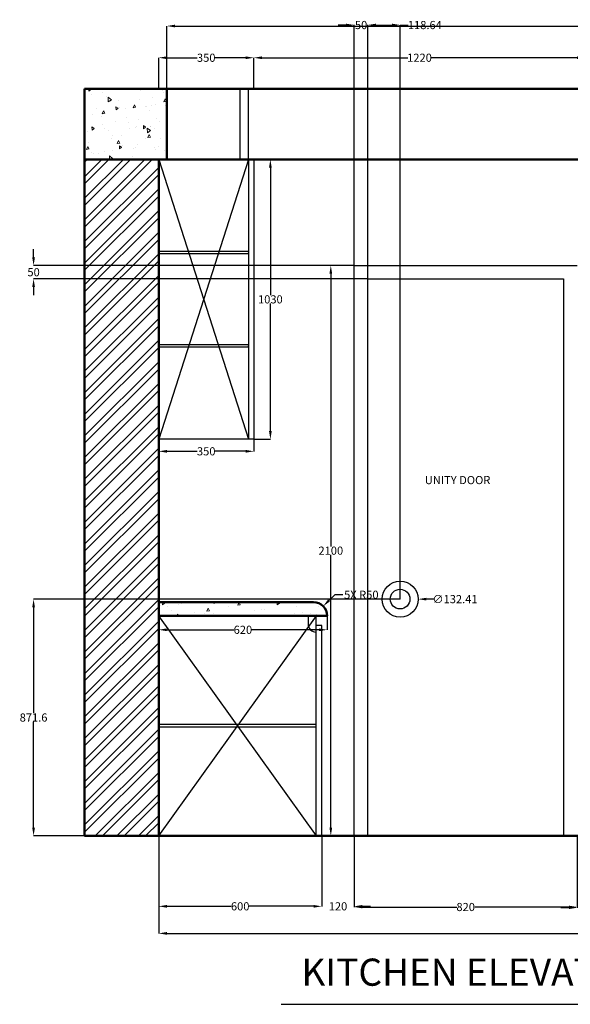
# Model space of a CAD drawing. Units: millimetres. Extents: x 26138 to 44889, y 15820 to 21179.
# Tile 5 of 8: x 35871 to 37898, y 15889 to 19513. Entities that reach past the tile are written whole.
import ezdxf

# ---------------------------------------------------------------- set-up
doc = ezdxf.new("R2010")
doc.units = ezdxf.units.MM
doc.header["$MEASUREMENT"] = 0
doc.header["$PDMODE"] = 3
for name, color, linetype, lineweight in [('A-ANNO-DIMS', 70, 'Continuous', 18), ('A-ANNO-SYMB', 1, 'Continuous', 18), ('A-ANNO-TEXT', 7, 'Continuous', 18), ('A-ELEV', 7, 'Continuous', 25), ('A-WALL', 1, 'Continuous', 50), ('A-WALL-PATT', 8, 'Continuous', 13)]:
    doc.layers.add(name, color=color, linetype=linetype, lineweight=lineweight)
doc.styles.get("Standard").update_dxf_attribs({"font": 'arial.ttf'})
doc.dimstyles.get("Standard").update_dxf_attribs({"dimtxt": 30, "dimasz": 30, "dimexe": 0.18, "dimexo": 0.0625, "dimgap": 0.09, "dimtad": 0, "dimtih": 1, "dimtoh": 1, "dimdec": 0, "dimzin": 0, "dimdsep": 46, "dimtxsty": 'Standard', "dimcen": 0.09, "dimadec": 0, "dimazin": 0, "dimtfac": 1, "dimtdec": 0, "dimtofl": 0, "dimtmove": 0, "dimatfit": 3, "dimfxl": 1, "dimtolj": 1, "dimtzin": 0, "dimarcsym": 0})

# ---------------------------------------------------------------- blocks, each defined once
blk = doc.blocks.new('*D71')
at = {"layer": 'A-ANNO-DIMS', "color": 0, "lineweight": -2, "transparency": 16777216}
for p, q in [((36382.5, 16508.7), (36382.5, 16249.3)), ((36982.5, 16508.7), (36982.5, 16249.3)), ((36412.5, 16249.5), (36649.3, 16249.5)), ((36952.5, 16249.5), (36715.8, 16249.5))]:
    blk.add_line(p, q, dxfattribs=at)
at = {"layer": 'A-ANNO-DIMS', "color": 0, "transparency": 16777216}
for points in [[(36412.5, 16254.5), (36412.5, 16244.5), (36382.5, 16249.5)], [(36952.5, 16254.5), (36952.5, 16244.5), (36982.5, 16249.5)]]:
    blk.add_solid(points, dxfattribs=at)
at = {"layer": 'Defpoints', "color": 0, "transparency": 16777216}
for p in [(36382.5, 16508.8), (36982.5, 16508.8), (36982.5, 16249.5)]:
    blk.add_point(p, dxfattribs=at)
at = {"layer": 'A-ANNO-DIMS', "color": 0, "transparency": 16777216, "insert": (36682.5, 16249.5), "char_height": 30, "attachment_point": 5}
blk.add_mtext('\\A1;600', dxfattribs=at)
blk = doc.blocks.new('*D72')
at = {"layer": 'A-ANNO-DIMS', "color": 0, "lineweight": -2, "transparency": 16777216}
for p, q in [((36982.5, 16508.7), (36982.5, 16249.3)), ((37102.5, 16508.7), (37102.5, 16249.3)), ((36952.5, 16249.5), (36922.5, 16249.5)), ((37132.5, 16249.5), (37162.5, 16249.5))]:
    blk.add_line(p, q, dxfattribs=at)
at = {"layer": 'A-ANNO-DIMS', "color": 0, "transparency": 16777216}
for points in [[(36952.5, 16254.5), (36952.5, 16244.5), (36982.5, 16249.5)], [(37132.5, 16254.5), (37132.5, 16244.5), (37102.5, 16249.5)]]:
    blk.add_solid(points, dxfattribs=at)
at = {"layer": 'Defpoints', "color": 0, "transparency": 16777216}
for p in [(36982.5, 16508.8), (37102.5, 16508.8), (37102.5, 16249.5)]:
    blk.add_point(p, dxfattribs=at)
at = {"layer": 'A-ANNO-DIMS', "color": 0, "transparency": 16777216, "insert": (37042.5, 16249.5), "char_height": 30, "attachment_point": 5}
blk.add_mtext('\\A1;120', dxfattribs=at)
blk = doc.blocks.new('*D73')
at = {"layer": 'A-ANNO-DIMS', "color": 0, "lineweight": -2, "transparency": 16777216}
for p, q in [((37102.5, 16508.7), (37102.5, 16246.8)), ((37922.5, 16508.7), (37922.5, 16246.8)), ((37132.5, 16247), (37479.3, 16247)), ((37892.5, 16247), (37545.7, 16247))]:
    blk.add_line(p, q, dxfattribs=at)
at = {"layer": 'A-ANNO-DIMS', "color": 0, "transparency": 16777216}
for points in [[(37132.5, 16252), (37132.5, 16242), (37102.5, 16247)], [(37892.5, 16252), (37892.5, 16242), (37922.5, 16247)]]:
    blk.add_solid(points, dxfattribs=at)
at = {"layer": 'Defpoints', "color": 0, "transparency": 16777216}
for p in [(37102.5, 16508.8), (37922.5, 16508.8), (37922.5, 16247)]:
    blk.add_point(p, dxfattribs=at)
at = {"layer": 'A-ANNO-DIMS', "color": 0, "transparency": 16777216, "insert": (37512.5, 16247), "char_height": 30, "attachment_point": 5}
blk.add_mtext('\\A1;820', dxfattribs=at)
blk = doc.blocks.new('*D74')
at = {"layer": 'A-ANNO-DIMS', "color": 0, "lineweight": -2, "transparency": 16777216}
for p, q in [((37922.5, 16508.7), (37922.5, 16244.3)), ((37952.5, 16508.7), (37952.5, 16244.3)), ((37892.5, 16244.5), (37862.5, 16244.5)), ((37982.5, 16244.5), (38012.5, 16244.5))]:
    blk.add_line(p, q, dxfattribs=at)
at = {"layer": 'A-ANNO-DIMS', "color": 0, "transparency": 16777216}
for points in [[(37892.5, 16249.5), (37892.5, 16239.5), (37922.5, 16244.5)], [(37982.5, 16249.5), (37982.5, 16239.5), (37952.5, 16244.5)]]:
    blk.add_solid(points, dxfattribs=at)
at = {"layer": 'Defpoints', "color": 0, "transparency": 16777216}
for p in [(37922.5, 16508.8), (37952.5, 16508.8), (37952.5, 16244.5)]:
    blk.add_point(p, dxfattribs=at)
at = {"layer": 'A-ANNO-DIMS', "color": 0, "transparency": 16777216, "insert": (38034.1, 16244.5), "char_height": 30, "attachment_point": 5}
blk.add_mtext('\\A1;30', dxfattribs=at)
blk = doc.blocks.new('*D85')
at = {"layer": 'A-ANNO-DIMS', "color": 0, "lineweight": -2, "transparency": 16777216}
for p, q in [((36382.5, 19258.8), (36382.5, 19373.3)), ((36412.5, 19373.2), (36524.4, 19373.2)), ((36702.5, 19373.2), (36590.7, 19373.2)), ((36732.5, 19258.8), (36732.5, 19373.3))]:
    blk.add_line(p, q, dxfattribs=at)
at = {"layer": 'A-ANNO-DIMS', "color": 0, "transparency": 16777216}
for points in [[(36412.5, 19378.2), (36412.5, 19368.2), (36382.5, 19373.2)], [(36702.5, 19378.2), (36702.5, 19368.2), (36732.5, 19373.2)]]:
    blk.add_solid(points, dxfattribs=at)
at = {"layer": 'Defpoints', "color": 0, "transparency": 16777216}
for p in [(36732.5, 19373.2), (36382.5, 19258.8), (36732.5, 19258.8)]:
    blk.add_point(p, dxfattribs=at)
at = {"layer": 'A-ANNO-DIMS', "color": 0, "transparency": 16777216, "insert": (36557.5, 19373.2), "char_height": 30, "attachment_point": 5}
blk.add_mtext('\\A1;350', dxfattribs=at)
blk = doc.blocks.new('*D86')
at = {"layer": 'A-ANNO-DIMS', "color": 0, "lineweight": -2, "transparency": 16777216}
for p, q in [((37016, 18608.8), (37015.9, 18608.8)), ((37016, 18578.8), (37016, 17574.2)), ((37016, 16538.8), (37016, 17543.4)), ((37016, 16508.8), (37015.9, 16508.8))]:
    blk.add_line(p, q, dxfattribs=at)
at = {"layer": 'A-ANNO-DIMS', "color": 0, "transparency": 16777216}
for points in [[(37011, 18578.8), (37021, 18578.8), (37016, 18608.8)], [(37011, 16538.8), (37021, 16538.8), (37016, 16508.8)]]:
    blk.add_solid(points, dxfattribs=at)
at = {"layer": 'Defpoints', "color": 0, "transparency": 16777216}
for p in [(37016, 18608.8), (37016, 18608.8), (37016, 16508.8)]:
    blk.add_point(p, dxfattribs=at)
at = {"layer": 'A-ANNO-DIMS', "color": 0, "transparency": 16777216, "insert": (37016, 17558.8), "char_height": 30, "attachment_point": 5}
blk.add_mtext('\\A1;2100', dxfattribs=at)
blk = doc.blocks.new('*D87')
at = {"layer": 'A-ANNO-DIMS', "color": 0, "lineweight": -2, "transparency": 16777216}
for p, q in [((36382.4, 17318.7), (36382.4, 17267.2)), ((37002.5, 17318.7), (37002.5, 17267.2)), ((36412.4, 17267.4), (36659.2, 17267.4)), ((36972.5, 17267.4), (36725.7, 17267.4))]:
    blk.add_line(p, q, dxfattribs=at)
at = {"layer": 'A-ANNO-DIMS', "color": 0, "transparency": 16777216}
for points in [[(36412.4, 17272.4), (36412.4, 17262.4), (36382.4, 17267.4)], [(36972.5, 17272.4), (36972.5, 17262.4), (37002.5, 17267.4)]]:
    blk.add_solid(points, dxfattribs=at)
at = {"layer": 'Defpoints', "color": 0, "transparency": 16777216}
for p in [(36382.4, 17318.8), (37002.5, 17318.8), (37002.5, 17267.4)]:
    blk.add_point(p, dxfattribs=at)
at = {"layer": 'A-ANNO-DIMS', "color": 0, "transparency": 16777216, "insert": (36692.5, 17267.4), "char_height": 30, "attachment_point": 5}
blk.add_mtext('\\A1;620', dxfattribs=at)
blk = doc.blocks.new('*D88')
at = {"layer": 'A-ANNO-DIMS', "color": 0, "lineweight": -2, "transparency": 16777216}
for p, q in [((36732.5, 19258.8), (36732.5, 19373.3)), ((36762.5, 19373.2), (37299.1, 19373.2)), ((37922.5, 19373.2), (37386, 19373.2)), ((37952.5, 19258.8), (37952.5, 19373.3))]:
    blk.add_line(p, q, dxfattribs=at)
at = {"layer": 'A-ANNO-DIMS', "color": 0, "transparency": 16777216}
for points in [[(36762.5, 19378.2), (36762.5, 19368.2), (36732.5, 19373.2)], [(37922.5, 19378.2), (37922.5, 19368.2), (37952.5, 19373.2)]]:
    blk.add_solid(points, dxfattribs=at)
at = {"layer": 'Defpoints', "color": 0, "transparency": 16777216}
for p in [(37952.5, 19373.2), (36732.5, 19258.8), (37952.5, 19258.8)]:
    blk.add_point(p, dxfattribs=at)
at = {"layer": 'A-ANNO-DIMS', "color": 0, "transparency": 16777216, "insert": (37342.5, 19373.2), "char_height": 30, "attachment_point": 5}
blk.add_mtext('\\A1;1220', dxfattribs=at)
blk = doc.blocks.new('*D92')
at = {"layer": 'A-ANNO-DIMS', "color": 0, "lineweight": -2, "transparency": 16777216}
for p, q in [((36382.5, 16509), (36382.5, 16149.6)), ((39582.5, 16508.7), (39582.5, 16149.6)), ((36412.5, 16149.8), (37937.7, 16149.8)), ((39552.5, 16149.8), (38027.4, 16149.8))]:
    blk.add_line(p, q, dxfattribs=at)
at = {"layer": 'A-ANNO-DIMS', "color": 0, "transparency": 16777216}
for points in [[(36412.5, 16154.8), (36412.5, 16144.8), (36382.5, 16149.8)], [(39552.5, 16154.8), (39552.5, 16144.8), (39582.5, 16149.8)]]:
    blk.add_solid(points, dxfattribs=at)
at = {"layer": 'Defpoints', "color": 0, "transparency": 16777216}
for p in [(36382.5, 16509), (39582.5, 16508.8), (39582.5, 16149.8)]:
    blk.add_point(p, dxfattribs=at)
at = {"layer": 'A-ANNO-DIMS', "color": 0, "transparency": 16777216, "insert": (37982.5, 16149.8), "char_height": 30, "attachment_point": 5}
blk.add_mtext('\\A1;3200', dxfattribs=at)
blk = doc.blocks.new('*D118')
at = {"layer": 'A-ANNO-DIMS', "color": 0, "lineweight": -2, "transparency": 16777216}
for p, q in [((36412.5, 19258.8), (36412.5, 19490)), ((36442.5, 19489.9), (38034.6, 19489.9)), ((39707.5, 19489.9), (38124.6, 19489.9)), ((39737.5, 19258.8), (39737.5, 19490))]:
    blk.add_line(p, q, dxfattribs=at)
at = {"layer": 'A-ANNO-DIMS', "color": 0, "transparency": 16777216}
for points in [[(36442.5, 19494.9), (36442.5, 19484.9), (36412.5, 19489.9)], [(39707.5, 19494.9), (39707.5, 19484.9), (39737.5, 19489.9)]]:
    blk.add_solid(points, dxfattribs=at)
at = {"layer": 'Defpoints', "color": 0, "transparency": 16777216}
for p in [(39737.5, 19489.9), (36412.5, 19258.8), (39737.5, 19258.8)]:
    blk.add_point(p, dxfattribs=at)
at = {"layer": 'A-ANNO-DIMS', "color": 0, "transparency": 16777216, "insert": (38079.6, 19489.9), "char_height": 30, "attachment_point": 5}
blk.add_mtext('\\A1;3325', dxfattribs=at)
blk = doc.blocks.new('*D123')
at = {"layer": 'A-ANNO-DIMS', "color": 0, "lineweight": -2, "transparency": 16777216}
for p, q in [((36732.6, 18998.8), (36793.7, 18998.8)), ((36793.6, 18968.8), (36793.6, 18499.2)), ((36793.6, 17998.8), (36793.6, 18468.3)), ((36732.6, 17968.8), (36793.7, 17968.8))]:
    blk.add_line(p, q, dxfattribs=at)
at = {"layer": 'A-ANNO-DIMS', "color": 0, "transparency": 16777216}
for points in [[(36788.6, 18968.8), (36798.6, 18968.8), (36793.6, 18998.8)], [(36788.6, 17998.8), (36798.6, 17998.8), (36793.6, 17968.8)]]:
    blk.add_solid(points, dxfattribs=at)
at = {"layer": 'Defpoints', "color": 0, "transparency": 16777216}
for p in [(36732.5, 18998.8), (36732.5, 17968.8), (36793.6, 17968.8)]:
    blk.add_point(p, dxfattribs=at)
at = {"layer": 'A-ANNO-DIMS', "color": 0, "transparency": 16777216, "insert": (36793.6, 18483.8), "char_height": 30, "attachment_point": 5}
blk.add_mtext('\\A1;1030', dxfattribs=at)
blk = doc.blocks.new('*D124')
at = {"layer": 'A-ANNO-DIMS', "color": 0, "lineweight": -2, "transparency": 16777216}
for p, q in [((36382.5, 17968.7), (36382.5, 17924.2)), ((36732.5, 17968.7), (36732.5, 17924.2)), ((36412.5, 17924.4), (36524.4, 17924.4)), ((36702.5, 17924.4), (36590.7, 17924.4))]:
    blk.add_line(p, q, dxfattribs=at)
at = {"layer": 'A-ANNO-DIMS', "color": 0, "transparency": 16777216}
for points in [[(36412.5, 17929.4), (36412.5, 17919.4), (36382.5, 17924.4)], [(36702.5, 17929.4), (36702.5, 17919.4), (36732.5, 17924.4)]]:
    blk.add_solid(points, dxfattribs=at)
at = {"layer": 'Defpoints', "color": 0, "transparency": 16777216}
for p in [(36382.5, 17968.8), (36732.5, 17968.8), (36732.5, 17924.4)]:
    blk.add_point(p, dxfattribs=at)
at = {"layer": 'A-ANNO-DIMS', "color": 0, "transparency": 16777216, "insert": (36557.5, 17924.4), "char_height": 30, "attachment_point": 5}
blk.add_mtext('\\A1;350', dxfattribs=at)
blk = doc.blocks.new('*D138')
at = {"layer": 'A-ANNO-DIMS', "color": 0, "lineweight": -2, "transparency": 16777216}
for p, q in [((37072.548484, 19493.567795), (37042.548484, 19493.567795)), ((37102.548484, 18608.828323), (37102.548484, 19493.747795)), ((37152.548484, 18558.828323), (37152.548484, 19493.747795)), ((37182.548484, 19493.567795), (37212.548484, 19493.567795))]:
    blk.add_line(p, q, dxfattribs=at)
at = {"layer": 'A-ANNO-DIMS', "color": 0, "transparency": 16777216}
for points in [[(37072.548484, 19498.567795), (37072.548484, 19488.567795), (37102.548484, 19493.567795)], [(37182.548484, 19498.567795), (37182.548484, 19488.567795), (37152.548484, 19493.567795)]]:
    blk.add_solid(points, dxfattribs=at)
at = {"layer": 'Defpoints', "color": 0, "transparency": 16777216}
for p in [(37152.548484, 19493.567795), (37102.548484, 18608.765823), (37152.548484, 18558.765823)]:
    blk.add_point(p, dxfattribs=at)
at = {"layer": 'A-ANNO-DIMS', "color": 0, "transparency": 16777216, "insert": (37127.548484, 19493.567795), "char_height": 30, "attachment_point": 5}
blk.add_mtext('\\A1;50', dxfattribs=at)
blk = doc.blocks.new('*D139')
at = {"layer": 'A-ANNO-DIMS', "color": 0, "lineweight": -2, "transparency": 16777216}
for p, q in [((35922.048484, 18638.765823), (35922.048484, 18668.765823)), ((37102.485984, 18608.765823), (35921.868484, 18608.765823)), ((37152.485984, 18558.765823), (35921.868484, 18558.765823)), ((35922.048484, 18528.765823), (35922.048484, 18498.765823))]:
    blk.add_line(p, q, dxfattribs=at)
at = {"layer": 'A-ANNO-DIMS', "color": 0, "transparency": 16777216}
for points in [[(35917.048484, 18638.765823), (35927.048484, 18638.765823), (35922.048484, 18608.765823)], [(35917.048484, 18528.765823), (35927.048484, 18528.765823), (35922.048484, 18558.765823)]]:
    blk.add_solid(points, dxfattribs=at)
at = {"layer": 'Defpoints', "color": 0, "transparency": 16777216}
for p in [(35922.048484, 18608.765823), (37102.548484, 18608.765823), (37152.548484, 18558.765823)]:
    blk.add_point(p, dxfattribs=at)
at = {"layer": 'A-ANNO-DIMS', "color": 0, "transparency": 16777216, "insert": (35922.048484, 18583.765823), "char_height": 30, "attachment_point": 5}
blk.add_mtext('\\A1;50', dxfattribs=at)
blk = doc.blocks.new('*D140')
at = {"layer": 'A-ANNO-DIMS', "color": 0, "lineweight": -2, "transparency": 16777216}
for p, q in [((37271.1, 17380.3), (35921.9, 17380.3)), ((35922, 17350.3), (35922, 16960)), ((35922, 16538.8), (35922, 16929.1)), ((37152.5, 16508.8), (35921.9, 16508.8))]:
    blk.add_line(p, q, dxfattribs=at)
at = {"layer": 'A-ANNO-DIMS', "color": 0, "transparency": 16777216}
for points in [[(35917, 17350.3), (35927, 17350.3), (35922, 17380.3)], [(35917, 16538.8), (35927, 16538.8), (35922, 16508.8)]]:
    blk.add_solid(points, dxfattribs=at)
at = {"layer": 'Defpoints', "color": 0, "transparency": 16777216}
for p in [(35922, 17380.3), (37271.2, 17380.3), (37152.5, 16508.8)]:
    blk.add_point(p, dxfattribs=at)
at = {"layer": 'A-ANNO-DIMS', "color": 0, "transparency": 16777216, "insert": (35922, 16944.5), "char_height": 30, "attachment_point": 5}
blk.add_mtext('\\A1;871.6', dxfattribs=at)
blk = doc.blocks.new('*D141')
at = {"layer": 'A-ANNO-DIMS', "color": 0, "lineweight": -2, "transparency": 16777216}
for p, q in [((37152.5, 18558.8), (37152.5, 19493.7)), ((37182.5, 19493.6), (37241.2, 19493.6)), ((37271.2, 17380.4), (37271.2, 19493.7)), ((37271.2, 19493.6), (37301.2, 19493.6))]:
    blk.add_line(p, q, dxfattribs=at)
at = {"layer": 'A-ANNO-DIMS', "color": 0, "transparency": 16777216}
for points in [[(37182.5, 19498.6), (37182.5, 19488.6), (37152.5, 19493.6)], [(37241.2, 19498.6), (37241.2, 19488.6), (37271.2, 19493.6)]]:
    blk.add_solid(points, dxfattribs=at)
at = {"layer": 'Defpoints', "color": 0, "transparency": 16777216}
for p in [(37271.2, 19493.6), (37152.5, 18558.8), (37271.2, 17380.3)]:
    blk.add_point(p, dxfattribs=at)
at = {"layer": 'A-ANNO-DIMS', "color": 0, "transparency": 16777216, "insert": (37362.1, 19493.6), "char_height": 30, "attachment_point": 5}
blk.add_mtext('\\A1;118.64', dxfattribs=at)
blk = doc.blocks.new('*D153')
at = {"layer": 'A-ANNO-DIMS', "color": 0, "lineweight": -2, "transparency": 16777216}
for p, q in [((37271.1, 17380.3), (37271.3, 17380.3)), ((37271.2, 17380.2), (37271.2, 17380.4)), ((37397.4, 17380.3), (37367.4, 17380.3))]:
    blk.add_line(p, q, dxfattribs=at)
at = {"layer": 'A-ANNO-DIMS', "color": 0, "transparency": 16777216}
blk.add_solid([(37367.4, 17385.3), (37367.4, 17375.3), (37337.4, 17380.3)], dxfattribs=at)
at = {"layer": 'Defpoints', "color": 0, "transparency": 16777216}
for p in [(37205, 17380.3), (37337.4, 17380.3)]:
    blk.add_point(p, dxfattribs=at)
at = {"layer": 'A-ANNO-DIMS', "color": 0, "transparency": 16777216, "insert": (37473.2, 17380.3), "char_height": 30, "attachment_point": 5}
blk.add_mtext('\\A1;∅132.41', dxfattribs=at)
blk = doc.blocks.new('*D154')
at = {"layer": 'A-ANNO-DIMS', "color": 0, "lineweight": -2, "transparency": 16777216}
for p, q in [((37030.3, 17396.5), (37009.1, 17375.3)), ((37060.3, 17396.5), (37030.3, 17396.5)), ((36952.5, 17318.7), (36952.5, 17318.9)), ((36952.5, 17318.8), (36952.6, 17318.8))]:
    blk.add_line(p, q, dxfattribs=at)
at = {"layer": 'A-ANNO-DIMS', "color": 0, "transparency": 16777216}
blk.add_solid([(37005.6, 17378.9), (37012.7, 17371.8), (36987.9, 17354.1)], dxfattribs=at)
at = {"layer": 'Defpoints', "color": 0, "transparency": 16777216}
for p in [(36987.9, 17354.1), (36952.5, 17318.8)]:
    blk.add_point(p, dxfattribs=at)
at = {"layer": 'A-ANNO-DIMS', "color": 0, "transparency": 16777216, "insert": (37128.4, 17396.5), "char_height": 30, "attachment_point": 5}
blk.add_mtext('\\A1;5X R50', dxfattribs=at)

msp = doc.modelspace()

# ---------------------------------------------------------------- hatches: boundary and pattern name
at = {"layer": 'A-WALL-PATT'}
h = msp.add_hatch(dxfattribs=at)
h.set_pattern_fill('AR-CONC', color=256, scale=16, angle=45)
h.set_pattern_definition([(95, (-15.19, -1836.28), (88.24832, 74.04913), [12, -132]), (40, (-15.19, -1836.28), (-100.79875, 69.4029), [9.6, -105.6]), (145.45144, (-7.83, -1830.11), (-12.55043, 143.45204), [10.19843, -112.18274]), (91.1842, (-37.81, -1813.65), (139.47094, 102.0182), [18, -198]), (141.63564, (-26.19, -1805.15), (-4.464, 215.95387), [15.29765, -168.2742]), (36.18416, (-37.81, -1813.65), (-4.464, 215.9539), [14.4, -158.4]), (66, (-20.84, -1808), (113.08345, 21.9812), [12, -132]), (11, (-20.84, -1808), (-54.51337, 109.56935), [9.6, -105.6]), (116.45144, (-11.42, -1806.17), (58.57008, 131.55054), [10.19843, -112.18274]), (82.5, (-15.186, -1836.282), (-36.28691, 39.03837), [0, -104.32, 0, -107.2, 0, -106]), (52.5, (-15.186, -1836.28), (-14.85967, 74.38551), [0, -61.12, 0, -101.92, 0, -40.4]), (12.5, (-40.416, -1861.51), (62.946907, 57.84332), [0, -40, 0, -124.8, 0, -165.6]), (2.5, (-51.73, -1872.826), (54.6544, 77.30557), [0, -52, 0, -82.88, 0, -117.6])])
h.paths.add_polyline_path([(36412.548, 19258.766), (36382.548, 19258.766), (36109.548, 19258.766), (36109.548, 18998.766), (36412.548, 18998.766)])
h = msp.add_hatch(dxfattribs=at)
h.set_pattern_fill('ANSI32', color=256, scale=150)
h.set_pattern_definition([(45, (-15.186, -1836.28), (-39.77476, 39.77476), []), (45, (11.33, -1836.28), (-39.77476, 39.77476), [])])
h.paths.add_polyline_path([(36109.548, 16508.766), (36382.548, 16508.766), (36382.548, 18998.766), (36109.548, 18998.766)])
h = msp.add_hatch(dxfattribs=at)
h.set_pattern_fill('AR-CONC', color=256, scale=16, angle=45)
h.set_pattern_definition([(95, (4.63, -1936.28), (88.24832, 74.04913), [12, -132]), (40, (4.63, -1936.28), (-100.79875, 69.4029), [9.6, -105.6]), (145.45144, (11.99, -1930.11), (-12.55043, 143.45204), [10.19843, -112.18274]), (91.1842, (-18, -1913.65), (139.47094, 102.0182), [18, -198]), (141.63564, (-6.37, -1905.15), (-4.464, 215.9539), [15.29765, -168.2742]), (36.18416, (-18, -1913.65), (-4.464, 215.9539), [14.4, -158.4]), (66, (-1.02, -1908), (113.08345, 21.9812), [12, -132]), (11, (-1.02, -1908), (-54.51337, 109.56935), [9.6, -105.6]), (116.45144, (8.4, -1906.17), (58.57008, 131.55054), [10.19843, -112.18274]), (82.5, (4.634, -1936.282), (-36.28691, 39.03837), [0, -104.32, 0, -107.2, 0, -106]), (52.5, (4.634, -1936.28), (-14.85967, 74.38551), [0, -61.12, 0, -101.92, 0, -40.4]), (12.5, (-20.596, -1961.51), (62.946907, 57.84332), [0, -40, 0, -124.8, 0, -165.6]), (2.5, (-31.91, -1972.826), (54.6544, 77.30557), [0, -52, 0, -82.88, 0, -117.6])])
edge = h.paths.add_edge_path()
edge.add_line((36952.548, 17368.766), (36382.368, 17368.766))
edge.add_line((36382.368, 17368.766), (36382.368, 17318.766))
edge.add_line((36382.368, 17318.766), (37002.548, 17318.766))
edge.add_arc((36952.548, 17318.766), 50, 0, 90)

# ---------------------------------------------------------------- linework, layer by layer
at = {"layer": 'A-ANNO-SYMB'}
for p in [(36712.548, 18655.432), (36712.548, 18312.099)]:
    msp.add_point(p, dxfattribs=at)
at = {"layer": 'A-ELEV'}
for p, q in [((36682.548, 18998.766), (36682.548, 19258.766)), ((36712.548, 18998.766), (36712.548, 19258.766)), ((36382.548, 18998.766), (36712.548, 17968.766)), ((36712.548, 18998.766), (36382.548, 17968.766)), ((36712.548, 18998.766), (36712.548, 17968.766)), ((36732.548, 18998.766), (36732.548, 17968.766)), ((36712.548, 18659.432), (36382.548, 18659.432)), ((36712.548, 18651.432), (36382.548, 18651.432)), ((37102.548, 16508.766), (37102.548, 18608.766)), ((37102.548, 18608.766), (37922.548, 18608.766)), ((37152.548, 18558.766), (37872.548, 18558.766)), ((37152.548, 16508.766), (37152.548, 18558.766)), ((37872.548, 18558.766), (37872.548, 16508.766)), ((36712.548, 18316.099), (36382.548, 18316.099)), ((36712.548, 18308.099), (36382.548, 18308.099)), ((36732.548, 17968.766), (36382.548, 17968.766)), ((36962.548, 17318.766), (36382.368, 16508.766)), ((36382.368, 17318.766), (36962.548, 16508.766)), ((36932.548, 17318.766), (36932.548, 17288.846)), ((36962.548, 16508.766), (36962.548, 17318.766)), ((36982.548, 17283.292), (36962.548, 17283.292)), ((36982.548, 16508.766), (36982.548, 17283.292)), ((36962.548, 16918.766), (36382.368, 16918.766)), ((36962.548, 16908.766), (36382.368, 16908.766)), ((36832.787, 15888.819), (38846.464, 15888.819))]:
    msp.add_line(p, q, dxfattribs=at)
for radius in [66.207, 36.207]:
    msp.add_circle((37271.187, 17380.331), radius, dxfattribs=at)
msp.add_arc((36962.548, 17288.846), 30, 180, 270, dxfattribs=at)
at = {"layer": 'A-WALL'}
for p, q in [((39737.548, 19258.766), (36109.548, 19258.766)), ((36109.548, 19258.766), (36109.548, 16508.766)), ((36412.548, 19258.766), (36412.548, 18998.766)), ((39582.548, 18998.766), (36109.548, 18998.766)), ((36382.548, 18998.766), (36382.548, 16508.766)), ((36952.548, 17368.766), (36382.368, 17368.766)), ((37002.548, 17318.766), (36382.368, 17318.766)), ((36109.548, 16508.766), (39737.548, 16508.766))]:
    msp.add_line(p, q, dxfattribs=at)
msp.add_arc((36952.548, 17318.766), 50, 0, 90, dxfattribs=at)

# ---------------------------------------------------------------- texts
at = {"layer": 'A-ANNO-TEXT'}
for s, height, p in [('UNITY DOOR', 30, (37361.99, 17803.568)), ('KITCHEN ELEVATION AT-B', 100, (36907.79, 15957.078))]:
    msp.add_text(s, height=height, dxfattribs=at).set_placement(p)

# ---------------------------------------------------------------- dimensions: what is measured, and where the dimension line sits
at = {"layer": 'A-ANNO-DIMS'}
dim = msp.add_linear_dim(base=(39737.548, 19489.858), p1=(36412.548, 19258.766), p2=(39737.548, 19258.766), dimstyle='Standard', override={"dimclrd": 0, "dimclre": 0, "dimclrt": 0}, dxfattribs=at)
dim.commit()
dim.dimension.update_dxf_attribs({"geometry": '*D118', "text_midpoint": (38079.614, 19489.858), "dimtype": 160})
for base, p1, p2, override, picture, middle in [((37152.548, 19493.568), (37102.548, 18608.766), (37152.548, 18558.766), {"dimdec": 0, "dimlfac": 1, "dimrnd": 0, "dimzin": 0, "dimdsep": 46, "dimlunit": 2}, '*D138', (37127.548, 19493.568)), ((37271.187, 19493.568), (37152.548, 18558.766), (37271.187, 17380.331), {"dimdec": 2, "dimlfac": 1, "dimrnd": 0, "dimzin": 0, "dimdsep": 46, "dimlunit": 2}, '*D141', (37362.075, 19493.568)), ((36732.548, 19373.162), (36382.548, 19258.766), (36732.548, 19258.766), {"dimclrd": 0, "dimclre": 0, "dimclrt": 0}, '*D85', (36557.548, 19373.162)), ((37952.548, 19373.162), (36732.548, 19258.766), (37952.548, 19258.766), {"dimclrd": 0, "dimclre": 0, "dimclrt": 0}, '*D88', (37342.548, 19373.162)), ((36732.548, 17924.409), (36382.548, 17968.766), (36732.548, 17968.766), {"dimclrd": 0, "dimclre": 0, "dimclrt": 0}, '*D124', (36557.548, 17924.409)), ((37002.548, 17267.374), (36382.368, 17318.766), (37002.548, 17318.766), {"dimclrd": 0, "dimclre": 0, "dimclrt": 0}, '*D87', (36692.458, 17267.374)), ((39582.548, 16149.822), (36382.548, 16509.017), (39582.548, 16508.766), {"dimclrd": 0, "dimclre": 0, "dimclrt": 0}, '*D92', (37982.548, 16149.822)), ((36982.548, 16249.467), (36382.548, 16508.766), (36982.548, 16508.766), {"dimclrd": 0, "dimclre": 0, "dimclrt": 0}, '*D71', (36682.548, 16249.467)), ((37102.548, 16249.467), (36982.548, 16508.766), (37102.548, 16508.766), {"dimclrd": 0, "dimclre": 0, "dimclrt": 0}, '*D72', (37042.548, 16249.467)), ((37922.548, 16246.967), (37102.548, 16508.766), (37922.548, 16508.766), {"dimclrd": 0, "dimclre": 0, "dimclrt": 0}, '*D73', (37512.548, 16246.967)), ((37952.548, 16244.467), (37922.548, 16508.766), (37952.548, 16508.766), {"dimclrd": 0, "dimclre": 0, "dimclrt": 0}, '*D74', (38034.064, 16244.467))]:
    dim = msp.add_linear_dim(base=base, p1=p1, p2=p2, dimstyle='Standard', override=override, dxfattribs=at)
    dim.commit()
    dim.dimension.update_dxf_attribs({"geometry": picture, "text_midpoint": middle})
for base, p1, p2, override, picture, middle in [((36793.563, 17968.766), (36732.548, 18998.766), (36732.548, 17968.766), {"dimclrd": 0, "dimclre": 0, "dimclrt": 0}, '*D123', (36793.563, 18483.766)), ((35922.048, 18608.766), (37152.548, 18558.766), (37102.548, 18608.766), {"dimdec": 0, "dimlfac": 1, "dimrnd": 0, "dimzin": 0, "dimdsep": 46, "dimlunit": 2}, '*D139', (35922.048, 18583.766)), ((35922.048, 17380.331), (37152.548, 16508.766), (37271.187, 17380.331), {"dimdec": 1, "dimlfac": 1, "dimrnd": 0, "dimzin": 0, "dimdsep": 46, "dimlunit": 2}, '*D140', (35922.048, 16944.549))]:
    dim = msp.add_linear_dim(base=base, p1=p1, p2=p2, angle=90, dimstyle='Standard', override=override, dxfattribs=at)
    dim.commit()
    dim.dimension.update_dxf_attribs({"geometry": picture, "text_midpoint": middle})
dim = msp.add_linear_dim(base=(37016.033, 18608.766), p1=(37016.033, 16508.766), p2=(37016.033, 18608.766), angle=90, dimstyle='Standard', override={"dimclrd": 0, "dimclre": 0, "dimclrt": 0}, dxfattribs=at)
dim.commit()
dim.dimension.update_dxf_attribs({"geometry": '*D86', "text_midpoint": (37016.033, 17558.766), "dimtype": 160})
dim = msp.add_radius_dim(center=(36952.548, 17318.766), mpoint=(36987.904, 17354.121), text='5X <>', dimstyle='Standard', override={"dimdec": 0, "dimlfac": 1, "dimrnd": 0, "dimzin": 0, "dimdsep": 46, "dimlunit": 2}, dxfattribs=at)
dim.commit()
dim.dimension.update_dxf_attribs({"geometry": '*D154', "text_midpoint": (37128.442, 17396.547)})
dim = msp.add_diameter_dim_2p(p1=(37204.98, 17380.332), p2=(37337.394, 17380.331), dimstyle='Standard', override={"dimdec": 2, "dimlfac": 1, "dimrnd": 0, "dimzin": 0, "dimdsep": 46, "dimlunit": 2}, dxfattribs=at)
dim.commit()
dim.dimension.update_dxf_attribs({"geometry": '*D153', "text_midpoint": (37397.394, 17380.331), "dimtype": 163})

doc.saveas('drawing.dxf')
